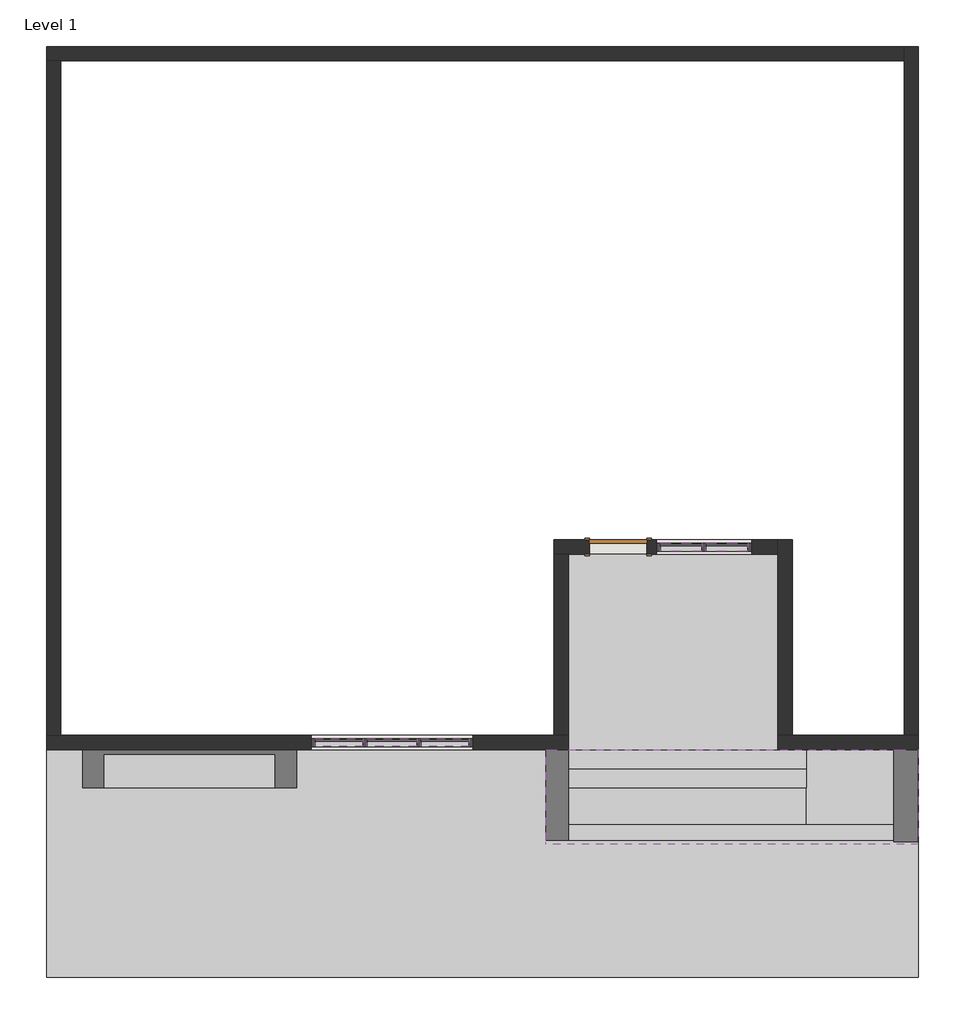
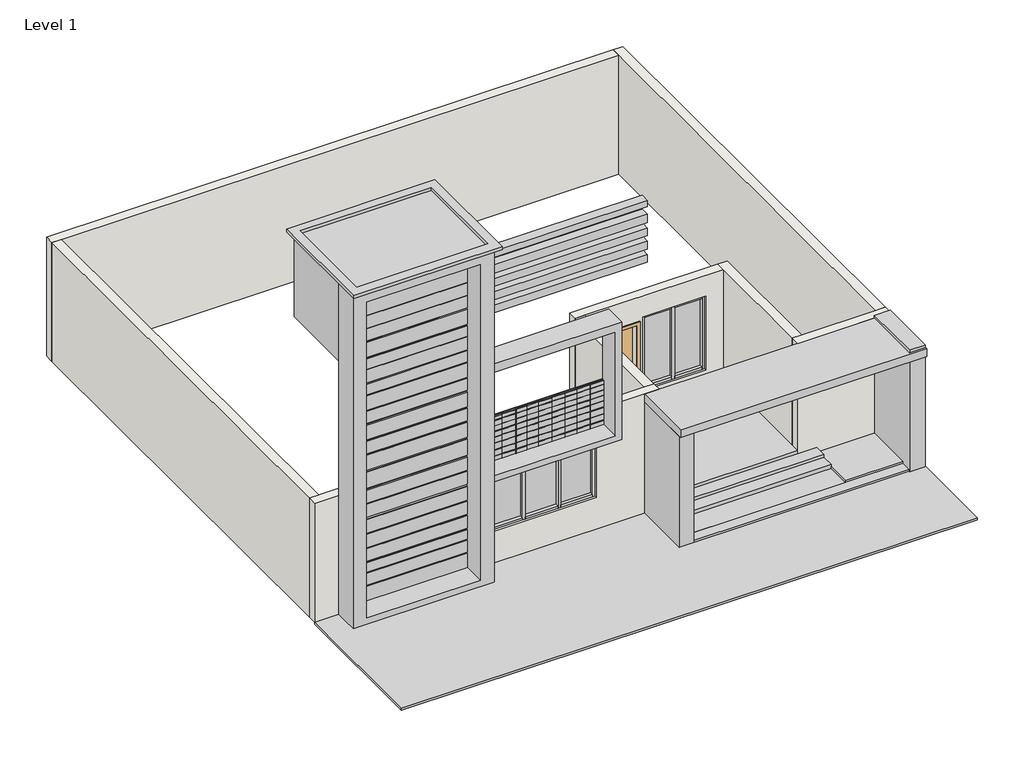
# One storey: 17 members, 8 walls, 5 plates, 4 proxies, 1 door.
"""IFC4 building model written with IfcOpenShell, lengths in millimetres."""

from ifc_helpers import new_model, si_unit, origin, origin_with_axes, place, context, project, spatial, polyline, outline, extrude, faceted_brep, transform, mapped, element, save
from components import generic_models_1_generic_models_1_ed8fc7ec, generic_models_3_generic_models_3_5e2efcd9, generic_models_4_generic_models_4_71681450, generic_models_6_generic_models_6_0c77f430, generic_models_6_generic_models_6_5a8cbb59, door_0ca8825f, member_46f5bc36, member_d36207d9, member_0a25ecd0, member_26ad134e, member_c33c434a, member_6a6f69b9, member_c9c2ffa2, system_panel_glazed_7ff316d0, system_panel_glazed_fe3e992a, system_panel_glazed_5e543223

model = new_model("IFC4")

# Units and contexts
model_context = context("Model", 3, world=origin())
ifc_project = project(units=[si_unit("LENGTHUNIT", "METRE", prefix="MILLI")], contexts=[model_context])

# Site, building, storey
site = spatial("IfcSite", under=ifc_project)
building = spatial("IfcBuilding", under=site)
storey = spatial("IfcBuildingStorey", under=building, Name="Level 1", Elevation=0.0)

# Proxies
placement = place(None, origin())
generic_models_1_generic_models_1_shape = generic_models_1_generic_models_1_ed8fc7ec(model_context)
element("IfcBuildingElementProxy", 1, Name="Generic Models 1 : Generic Models 1", ObjectType="Generic Models 1 : Generic Models 1", at=placement, inside=storey, context=model_context, shape_type="MappedRepresentation", body=[
    mapped(generic_models_1_generic_models_1_shape, transform((0.0, 0.0, 0.0), x_axis=(1.0, 0.0, 0.0), y_axis=(0.0, 1.0, 0.0), z_axis=(0.0, 0.0, 1.0))),
])
generic_models_3_generic_models_3_shape = generic_models_3_generic_models_3_5e2efcd9(model_context)
element("IfcBuildingElementProxy", 2, Name="Generic Models 3 : Generic Models 3", ObjectType="Generic Models 3 : Generic Models 3", at=placement, inside=storey, context=model_context, shape_type="MappedRepresentation", body=[
    mapped(generic_models_3_generic_models_3_shape, transform((0.0, 0.0, 0.0), x_axis=(1.0, 0.0, 0.0), y_axis=(0.0, 1.0, 0.0), z_axis=(0.0, 0.0, 1.0))),
])
generic_models_4_generic_models_4_shape = generic_models_4_generic_models_4_71681450(model_context)
element("IfcBuildingElementProxy", 3, Name="Generic Models 4 : Generic Models 4", ObjectType="Generic Models 4 : Generic Models 4", at=placement, inside=storey, context=model_context, shape_type="MappedRepresentation", body=[
    mapped(generic_models_4_generic_models_4_shape, transform((0.0, 0.0, 0.0), x_axis=(1.0, 0.0, 0.0), y_axis=(0.0, 1.0, 0.0), z_axis=(0.0, 0.0, 1.0))),
])
generic_models_6_generic_models_6_shape = generic_models_6_generic_models_6_0c77f430(model_context)
generic_models_6_generic_models_6_2_shape = generic_models_6_generic_models_6_5a8cbb59(model_context)
element("IfcBuildingElementProxy", 4, Name="Generic Models 6 : Generic Models 6", ObjectType="Generic Models 6 : Generic Models 6", at=placement, inside=storey, context=model_context, shape_type="MappedRepresentation", body=[
    mapped(generic_models_6_generic_models_6_shape, transform((0.0, 0.0, 0.0), x_axis=(1.0, 0.0, 0.0), y_axis=(0.0, 1.0, 0.0), z_axis=(0.0, 0.0, 1.0))),
    mapped(generic_models_6_generic_models_6_2_shape, transform((0.0, 0.0, 0.0), x_axis=(1.0, 0.0, 0.0), y_axis=(0.0, 1.0, 0.0), z_axis=(0.0, 0.0, 1.0))),
])

# Door
door_shape = door_0ca8825f(model_context)
element("IfcDoor", 5, ObjectType="Single-Flush : 36\" x 84\"", at=placement, inside=storey, context=model_context, shape_type="MappedRepresentation", body=[
    mapped(door_shape, transform((-9378.8831929, -7047.9592534, 228.6), x_axis=(1.0, 0.0, 0.0), y_axis=(0.0, 1.0, 0.0), z_axis=(0.0, 0.0, 1.0))),
])

# Members
member_shape = member_46f5bc36(model_context)
element("IfcMember", 6, ObjectType="Rectangular Mullion : 2.5\" x 5\" rectangular", at=placement, inside=storey, context=model_context, shape_type="MappedRepresentation", body=[
    mapped(member_shape, transform((-12534.8331929, -10172.1592534, 813.2979784), x_axis=(0.0, 0.0, -1.0), y_axis=(0.0, -1.0, 0.0), z_axis=(-1.0, 0.0, 0.0))),
])
element("IfcMember", 7, ObjectType="Rectangular Mullion : 2.5\" x 5\" rectangular", at=placement, inside=storey, context=model_context, shape_type="MappedRepresentation", body=[
    mapped(member_shape, transform((-14230.2831929, -10172.1592534, 813.2979784), x_axis=(0.0, 0.0, -1.0), y_axis=(0.0, -1.0, 0.0), z_axis=(-1.0, 0.0, 0.0))),
])
member_2_shape = member_d36207d9(model_context)
element("IfcMember", 8, ObjectType="Rectangular Mullion : 2.5\" x 5\" rectangular", at=placement, inside=storey, context=model_context, shape_type="MappedRepresentation", body=[
    mapped(member_2_shape, transform((-13398.4331929, -10172.1592534, 813.2979784), x_axis=(0.0, 0.0, -1.0), y_axis=(0.0, -1.0, 0.0), z_axis=(-1.0, 0.0, 0.0))),
])
member_3_shape = member_0a25ecd0(model_context)
element("IfcMember", 9, ObjectType="Rectangular Mullion : 2.5\" x 5\" rectangular", at=placement, inside=storey, context=model_context, shape_type="MappedRepresentation", body=[
    mapped(member_3_shape, transform((-13430.1831929, -10172.1592534, 813.2979784), x_axis=(1.0, 0.0, 0.0), y_axis=(0.0, -1.0, 0.0), z_axis=(0.0, 0.0, -1.0))),
])
element("IfcMember", 10, ObjectType="Rectangular Mullion : 2.5\" x 5\" rectangular", at=placement, inside=storey, context=model_context, shape_type="MappedRepresentation", body=[
    mapped(member_3_shape, transform((-12566.5831929, -10172.1592534, 813.2979784), x_axis=(1.0, 0.0, 0.0), y_axis=(0.0, -1.0, 0.0), z_axis=(0.0, 0.0, -1.0))),
])
element("IfcMember", 11, ObjectType="Rectangular Mullion : 2.5\" x 5\" rectangular", at=placement, inside=storey, context=model_context, shape_type="MappedRepresentation", body=[
    mapped(member_2_shape, transform((-12598.3331929, -10172.1592534, 2506.9923672), x_axis=(0.0, 0.0, 1.0), y_axis=(0.0, -1.0, 0.0), z_axis=(1.0, 0.0, 0.0))),
])
element("IfcMember", 12, ObjectType="Rectangular Mullion : 2.5\" x 5\" rectangular", at=placement, inside=storey, context=model_context, shape_type="MappedRepresentation", body=[
    mapped(member_shape, transform((-13461.9331929, -10172.1592534, 2506.9923672), x_axis=(0.0, 0.0, 1.0), y_axis=(0.0, -1.0, 0.0), z_axis=(1.0, 0.0, 0.0))),
])
element("IfcMember", 13, ObjectType="Rectangular Mullion : 2.5\" x 5\" rectangular", at=placement, inside=storey, context=model_context, shape_type="MappedRepresentation", body=[
    mapped(member_shape, transform((-11766.4831929, -10172.1592534, 2506.9923672), x_axis=(0.0, 0.0, 1.0), y_axis=(0.0, -1.0, 0.0), z_axis=(1.0, 0.0, 0.0))),
])
member_4_shape = member_26ad134e(model_context)
element("IfcMember", 14, ObjectType="Rectangular Mullion : 2.5\" x 5\" rectangular", at=placement, inside=storey, context=model_context, shape_type="MappedRepresentation", body=[
    mapped(member_4_shape, transform((-14293.7831929, -10172.1592534, 2506.9923672), x_axis=(-1.0, 0.0, 0.0), y_axis=(0.0, -1.0, 0.0), z_axis=(0.0, 0.0, 1.0))),
])
element("IfcMember", 15, ObjectType="Rectangular Mullion : 2.5\" x 5\" rectangular", at=placement, inside=storey, context=model_context, shape_type="MappedRepresentation", body=[
    mapped(member_4_shape, transform((-11702.9831929, -10172.1592534, 813.2979784), x_axis=(1.0, 0.0, 0.0), y_axis=(0.0, -1.0, 0.0), z_axis=(0.0, 0.0, -1.0))),
])
member_5_shape = member_c33c434a(model_context)
element("IfcMember", 16, ObjectType="Rectangular Mullion : 2.5\" x 5\" rectangular", at=placement, inside=storey, context=model_context, shape_type="MappedRepresentation", body=[
    mapped(member_5_shape, transform((-8039.0331929, -7047.9592534, 2507.9918264), x_axis=(0.0, 0.0, 1.0), y_axis=(0.0, -1.0, 0.0), z_axis=(1.0, 0.0, 0.0))),
])
element("IfcMember", 17, ObjectType="Rectangular Mullion : 2.5\" x 5\" rectangular", at=placement, inside=storey, context=model_context, shape_type="MappedRepresentation", body=[
    mapped(member_5_shape, transform((-7308.7831929, -7047.9592534, 2507.9918264), x_axis=(0.0, 0.0, 1.0), y_axis=(0.0, -1.0, 0.0), z_axis=(1.0, 0.0, 0.0))),
])
member_6_shape = member_6a6f69b9(model_context)
element("IfcMember", 18, ObjectType="Rectangular Mullion : 2.5\" x 5\" rectangular", at=placement, inside=storey, context=model_context, shape_type="MappedRepresentation", body=[
    mapped(member_6_shape, transform((-8007.2831929, -7047.9592534, 620.7008162), x_axis=(1.0, 0.0, 0.0), y_axis=(0.0, -1.0, 0.0), z_axis=(0.0, 0.0, -1.0))),
])
element("IfcMember", 19, ObjectType="Rectangular Mullion : 2.5\" x 5\" rectangular", at=placement, inside=storey, context=model_context, shape_type="MappedRepresentation", body=[
    mapped(member_5_shape, transform((-7975.5331929, -7047.9592534, 620.7008162), x_axis=(0.0, 0.0, -1.0), y_axis=(0.0, -1.0, 0.0), z_axis=(-1.0, 0.0, 0.0))),
])
element("IfcMember", 20, ObjectType="Rectangular Mullion : 2.5\" x 5\" rectangular", at=placement, inside=storey, context=model_context, shape_type="MappedRepresentation", body=[
    mapped(member_5_shape, transform((-8705.7831929, -7047.9592534, 620.7008162), x_axis=(0.0, 0.0, -1.0), y_axis=(0.0, -1.0, 0.0), z_axis=(-1.0, 0.0, 0.0))),
])
member_7_shape = member_c9c2ffa2(model_context)
element("IfcMember", 21, ObjectType="Rectangular Mullion : 2.5\" x 5\" rectangular", at=placement, inside=storey, context=model_context, shape_type="MappedRepresentation", body=[
    mapped(member_7_shape, transform((-8769.2831929, -7047.9592534, 2507.9918264), x_axis=(-1.0, 0.0, 0.0), y_axis=(0.0, -1.0, 0.0), z_axis=(0.0, 0.0, 1.0))),
])
element("IfcMember", 22, ObjectType="Rectangular Mullion : 2.5\" x 5\" rectangular", at=placement, inside=storey, context=model_context, shape_type="MappedRepresentation", body=[
    mapped(member_7_shape, transform((-7245.2831929, -7047.9592534, 620.7008162), x_axis=(1.0, 0.0, 0.0), y_axis=(0.0, -1.0, 0.0), z_axis=(0.0, 0.0, -1.0))),
])

# Plates
system_panel_glazed_shape = system_panel_glazed_7ff316d0(model_context)
element("IfcPlate", 23, ObjectType="System Panel : Glazed", at=placement, inside=storey, context=model_context, shape_type="MappedRepresentation", body=[
    mapped(system_panel_glazed_shape, transform((-13846.1081929, -10172.1592534, 876.7979784), x_axis=(1.0, 0.0, 0.0), y_axis=(0.0, 1.0, 0.0), z_axis=(0.0, 0.0, 1.0))),
])
element("IfcPlate", 24, ObjectType="System Panel : Glazed", at=placement, inside=storey, context=model_context, shape_type="MappedRepresentation", body=[
    mapped(system_panel_glazed_shape, transform((-12150.6581929, -10172.1592534, 876.7979784), x_axis=(1.0, 0.0, 0.0), y_axis=(0.0, 1.0, 0.0), z_axis=(0.0, 0.0, 1.0))),
])
system_panel_glazed_2_shape = system_panel_glazed_fe3e992a(model_context)
element("IfcPlate", 25, ObjectType="System Panel : Glazed", at=placement, inside=storey, context=model_context, shape_type="MappedRepresentation", body=[
    mapped(system_panel_glazed_2_shape, transform((-12998.3831929, -10172.1592534, 876.7979784), x_axis=(1.0, 0.0, 0.0), y_axis=(0.0, 1.0, 0.0), z_axis=(0.0, 0.0, 1.0))),
])
system_panel_glazed_3_shape = system_panel_glazed_5e543223(model_context)
element("IfcPlate", 26, ObjectType="System Panel : Glazed", at=placement, inside=storey, context=model_context, shape_type="MappedRepresentation", body=[
    mapped(system_panel_glazed_3_shape, transform((-8372.4081929, -7047.9592534, 684.2008162), x_axis=(1.0, 0.0, 0.0), y_axis=(0.0, 1.0, 0.0), z_axis=(0.0, 0.0, 1.0))),
])
element("IfcPlate", 27, ObjectType="System Panel : Glazed", at=placement, inside=storey, context=model_context, shape_type="MappedRepresentation", body=[
    mapped(system_panel_glazed_3_shape, transform((-7642.1581929, -7047.9592534, 684.2008162), x_axis=(1.0, 0.0, 0.0), y_axis=(0.0, 1.0, 0.0), z_axis=(0.0, 0.0, 1.0))),
])

# Walls
element("IfcWall", 28, ObjectType="9\"", at=placement, inside=storey, context=model_context, shape_type="Brep", body=[
    faceted_brep([(-18522.8831929, -10286.4592534, 0.0), (-10178.9831929, -10286.4592534, 0.0), (-10178.9831929, -10286.4592534, 3048.0), (-18522.8831929, -10286.4592534, 3048.0), (-14293.7831929, -10286.4592534, 813.2979784), (-14293.7831929, -10286.4592534, 2506.9923672), (-11702.9831929, -10286.4592534, 2506.9923672), (-11702.9831929, -10286.4592534, 813.2979784), (-10178.9831929, -10057.8592534, 0.0), (-10407.5831929, -10057.8592534, 0.0), (-18294.2831929, -10057.8592534, 0.0), (-18522.8831929, -10057.8592534, 0.0), (-18522.8831929, -10057.8592534, 3048.0), (-18294.2831929, -10057.8592534, 3048.0), (-10407.5831929, -10057.8592534, 3048.0), (-10178.9831929, -10057.8592534, 3048.0), (-14293.7831929, -10057.8592534, 2506.9923672), (-14293.7831929, -10057.8592534, 813.2979784), (-11702.9831929, -10057.8592534, 813.2979784), (-11702.9831929, -10057.8592534, 2506.9923672)], [[[0, 1, 2, 3], [4, 5, 6, 7]], [[8, 9, 10, 11, 12, 13, 14, 15], [16, 17, 18, 19]], [[1, 0, 11, 10, 9, 8]], [[2, 1, 8, 15]], [[3, 2, 15, 14, 13, 12]], [[0, 3, 12, 11]], [[4, 17, 16, 5]], [[5, 16, 19, 6]], [[6, 19, 18, 7]], [[17, 4, 7, 18]]]),
])
element("IfcWall", 29, ObjectType="9\"", at=placement, inside=storey, context=model_context, shape_type="Brep", body=[
    faceted_brep([(-4578.2831929, -10057.8592534, 0.0), (-4578.2831929, 953.0407466, 0.0), (-4578.2831929, 953.0407466, 3048.0), (-4578.2831929, -10057.8592534, 3048.0), (-4806.8831929, -10057.8592534, 0.0), (-4806.8831929, -10057.8592534, 3048.0), (-4806.8831929, 724.4407466, 3048.0), (-4806.8831929, 953.0407466, 3048.0), (-4806.8831929, 953.0407466, 0.0), (-4806.8831929, 724.4407466, 0.0)], [[[0, 1, 2, 3]], [[4, 5, 6, 7, 8, 9]], [[1, 0, 4, 9, 8]], [[3, 2, 7, 6, 5]], [[0, 3, 5, 4]], [[2, 1, 8, 7]]]),
])
element("IfcWall", 30, ObjectType="9\"", at=placement, inside=storey, context=model_context, shape_type="Brep", body=[
    faceted_brep([(-4806.8831929, 953.0407466, 0.0), (-18522.8831929, 953.0407466, 0.0), (-18522.8831929, 953.0407466, 3048.0), (-4806.8831929, 953.0407466, 3048.0), (-4806.8831929, 724.4407466, 0.0), (-4806.8831929, 724.4407466, 3048.0), (-18294.2831929, 724.4407466, 3048.0), (-18522.8831929, 724.4407466, 3048.0), (-18522.8831929, 724.4407466, 0.0), (-18294.2831929, 724.4407466, 0.0)], [[[0, 1, 2, 3]], [[4, 5, 6, 7, 8, 9]], [[1, 0, 4, 9, 8]], [[3, 2, 7, 6, 5]], [[0, 3, 5, 4]], [[2, 1, 8, 7]]]),
])
element("IfcWall", 31, ObjectType="9\"", at=placement, inside=storey, context=model_context, shape_type="SweptSolid", body=[
    extrude(outline(polyline([(-18522.8831929, -10057.8592534), (-18522.8831929, 724.4407466), (-18294.2831929, 724.4407466), (-18294.2831929, -10057.8592534), (-18522.8831929, -10057.8592534)])), origin_with_axes(), (0.0, 0.0, 1.0), 3048.0),
])
element("IfcWall", 32, ObjectType="9\"", at=placement, inside=storey, context=model_context, shape_type="Brep", body=[
    faceted_brep([(-6597.5831929, -10057.8592534, 0.0), (-6597.5831929, -6933.6592534, 0.0), (-6597.5831929, -6933.6592534, 3048.0), (-6597.5831929, -10057.8592534, 3048.0), (-6826.1831929, -10057.8592534, 0.0), (-6826.1831929, -10057.8592534, 3048.0), (-6826.1831929, -7162.2592534, 3048.0), (-6826.1831929, -6933.6592534, 3048.0), (-6826.1831929, -6933.6592534, 0.0), (-6826.1831929, -7162.2592534, 0.0)], [[[0, 1, 2, 3]], [[4, 5, 6, 7, 8, 9]], [[1, 0, 4, 9, 8]], [[3, 2, 7, 6, 5]], [[0, 3, 5, 4]], [[2, 1, 8, 7]]]),
])
element("IfcWall", 33, ObjectType="9\"", at=placement, inside=storey, context=model_context, shape_type="Brep", body=[
    faceted_brep([(-6826.1831929, -6933.6592534, 0.0), (-10407.5831929, -6933.6592534, 0.0), (-10407.5831929, -6933.6592534, 3048.0), (-6826.1831929, -6933.6592534, 3048.0), (-9836.0831929, -6933.6592534, 228.6), (-8921.6831929, -6933.6592534, 228.6), (-8921.6831929, -6933.6592534, 2362.2), (-9836.0831929, -6933.6592534, 2362.2), (-8769.2831929, -6933.6592534, 2507.9918264), (-8769.2831929, -6933.6592534, 620.7008162), (-7245.2831929, -6933.6592534, 620.7008162), (-7245.2831929, -6933.6592534, 2507.9918264), (-10407.5831929, -7162.2592534, 0.0), (-10178.9831929, -7162.2592534, 0.0), (-6826.1831929, -7162.2592534, 0.0), (-6826.1831929, -7162.2592534, 3048.0), (-10178.9831929, -7162.2592534, 3048.0), (-10407.5831929, -7162.2592534, 3048.0), (-8921.6831929, -7162.2592534, 228.6), (-9836.0831929, -7162.2592534, 228.6), (-9836.0831929, -7162.2592534, 2362.2), (-8921.6831929, -7162.2592534, 2362.2), (-8769.2831929, -7162.2592534, 620.7008162), (-8769.2831929, -7162.2592534, 2507.9918264), (-7245.2831929, -7162.2592534, 2507.9918264), (-7245.2831929, -7162.2592534, 620.7008162)], [[[0, 1, 2, 3], [4, 5, 6, 7], [8, 9, 10, 11]], [[12, 13, 14, 15, 16, 17], [18, 19, 20, 21], [22, 23, 24, 25]], [[1, 0, 14, 13, 12]], [[3, 2, 17, 16, 15]], [[0, 3, 15, 14]], [[2, 1, 12, 17]], [[5, 4, 19, 18]], [[6, 5, 18, 21]], [[7, 6, 21, 20]], [[4, 7, 20, 19]], [[22, 9, 8, 23]], [[23, 8, 11, 24]], [[24, 11, 10, 25]], [[9, 22, 25, 10]]]),
])
element("IfcWall", 34, ObjectType="9\"", at=placement, inside=storey, context=model_context, shape_type="SweptSolid", body=[
    extrude(outline(polyline([(-10407.5831929, -10057.8592534), (-10407.5831929, -7162.2592534), (-10178.9831929, -7162.2592534), (-10178.9831929, -10057.8592534), (-10407.5831929, -10057.8592534)])), origin_with_axes(), (0.0, 0.0, 1.0), 3048.0),
])
element("IfcWall", 35, ObjectType="9\"", at=placement, inside=storey, context=model_context, shape_type="Brep", body=[
    faceted_brep([(-6826.1831929, -10286.4592534, 0.0), (-4578.2831929, -10286.4592534, 0.0), (-4578.2831929, -10286.4592534, 3048.0), (-6826.1831929, -10286.4592534, 3048.0), (-6826.1831929, -10057.8592534, 0.0), (-6826.1831929, -10057.8592534, 3048.0), (-6597.5831929, -10057.8592534, 3048.0), (-4806.8831929, -10057.8592534, 3048.0), (-4578.2831929, -10057.8592534, 3048.0), (-4578.2831929, -10057.8592534, 0.0), (-4806.8831929, -10057.8592534, 0.0), (-6597.5831929, -10057.8592534, 0.0)], [[[0, 1, 2, 3]], [[4, 5, 6, 7, 8, 9, 10, 11]], [[1, 0, 4, 11, 10, 9]], [[3, 2, 8, 7, 6, 5]], [[0, 3, 5, 4]], [[2, 1, 9, 8]]]),
])

save(model, "model.ifc")

# Revit data of these elements
# Type "Single-Flush : 36\" x 84\""
#   Type Mark = "1"
#   Construction Type Id = "MDOOR"
#   Assembly Code = "C1020"
#   Analytic Construction = "Metal"
#   Thickness = 0' - 2"
#   Heat Transfer Coefficient (U) = 0.651978 BTU/(h·ft²·°F)
#   Height = 7' - 0"
#   Trim Projection Ext = 0' - 1"
#   Trim Projection Int = 0' - 1"
#   Trim Width = 0' - 3"
#   Width = 3' - 0"
#   Define Thermal Properties by = 1
#   Define Thermal Properties by = 1
#   Door Material = Door - Panel
#   Frame Material = Door - Frame
#   Visual Light Transmittance = 0
#   Solar Heat Gain Coefficient = 0
#   Function = (empty or 0)
#   Wall Closure = (empty or 0)
# Type "Rectangular Mullion : 2.5\" x 5\" rectangular"
#   built-in parameter 1007304 = 0.416667 (stored number, unit not read)
#   built-in parameter 1007301 = 0.104167 (stored number, unit not read)
#   built-in parameter 1007300 = 0.104167 (stored number, unit not read)
# Type "System Panel : Glazed"
#   Construction Type Id = "GSP4R"
#   Analytic Construction = "1/8 in Pilkington single glazing"
#   Visual Light Transmittance = 0.9
#   Solar Heat Gain Coefficient = 0.86
#   Heat Transfer Coefficient (U) = 1.18115 BTU/(h·ft²·°F)
#   Define Thermal Properties by = 1
# Type "9\""
#   Assembly Code = "B2010"
#   Layers, outside or top first: 0' - 9" no material (function 1)
# Element 1 (IfcBuildingElementProxy, "Generic Models 1 : Generic Models 1")
#   Phase Created = New Construction
# Element 2 (IfcBuildingElementProxy, "Generic Models 3 : Generic Models 3")
#   Phase Created = New Construction
# Element 3 (IfcBuildingElementProxy, "Generic Models 4 : Generic Models 4")
#   Phase Created = New Construction
#   Materials on its faces: "Tile, Porcelain, 4in"
# Element 4 (IfcBuildingElementProxy, "Generic Models 6 : Generic Models 6")
#   Phase Created = New Construction
# Element 5 (IfcDoor, "Single-Flush : 36\" x 84\"")
#   Phase Created = New Construction
#   Materials on its faces: "Door - Frame", "Door - Panel"
# Elements 6, 7, 8, 9, 10, 11, 12, 13, 14, 15, 16, 17, 18, 19, 20, 21, 22 (IfcMember, "Rectangular Mullion : 2.5\" x 5\" rectangular")
#   Phase Created = New Construction
#   Materials on its faces: "Aluminum"
# Elements 23, 24, 25, 26, 27 (IfcPlate, "System Panel : Glazed")
#   Phase Created = New Construction
#   Materials on its faces: "Glass"
# Elements 28, 29, 30, 31, 32, 33, 34, 35 (IfcWall, "9\"")
#   Top Offset = 0' - 0"
#   Base Offset = 0' - 0"
#   Unconnected Height = 10' - 0"
#   wall height = 10' - 0"
#   Phase Created = New Construction
#   Base Constraint = Level 1
#   Materials on its faces: "Default Wall"
# Materials
#   "Door - Panel": class "Wood", colour RGB 210 159 95, transparency 0, Cost = 0
#   "Door - Frame": colour RGB 118 70 51, transparency 0, Cost = 0
#   "Tile, Porcelain, 4in": class "Generic", colour RGB 89 87 158, transparency 0, Description = "Porcelain tile, 4\", white", Cost = 0
#   "Aluminum": class "Metal", colour RGB 247 247 247, transparency 0, Description = "Aluminum 6061", Cost = 0
#   "Glass": class "Glass", colour RGB 0 128 192, transparency 0.75, Description = "Soda Lime Glass", Cost = 0
#   "Default Wall": colour RGB 128 128 128, transparency 0, Cost = 0
